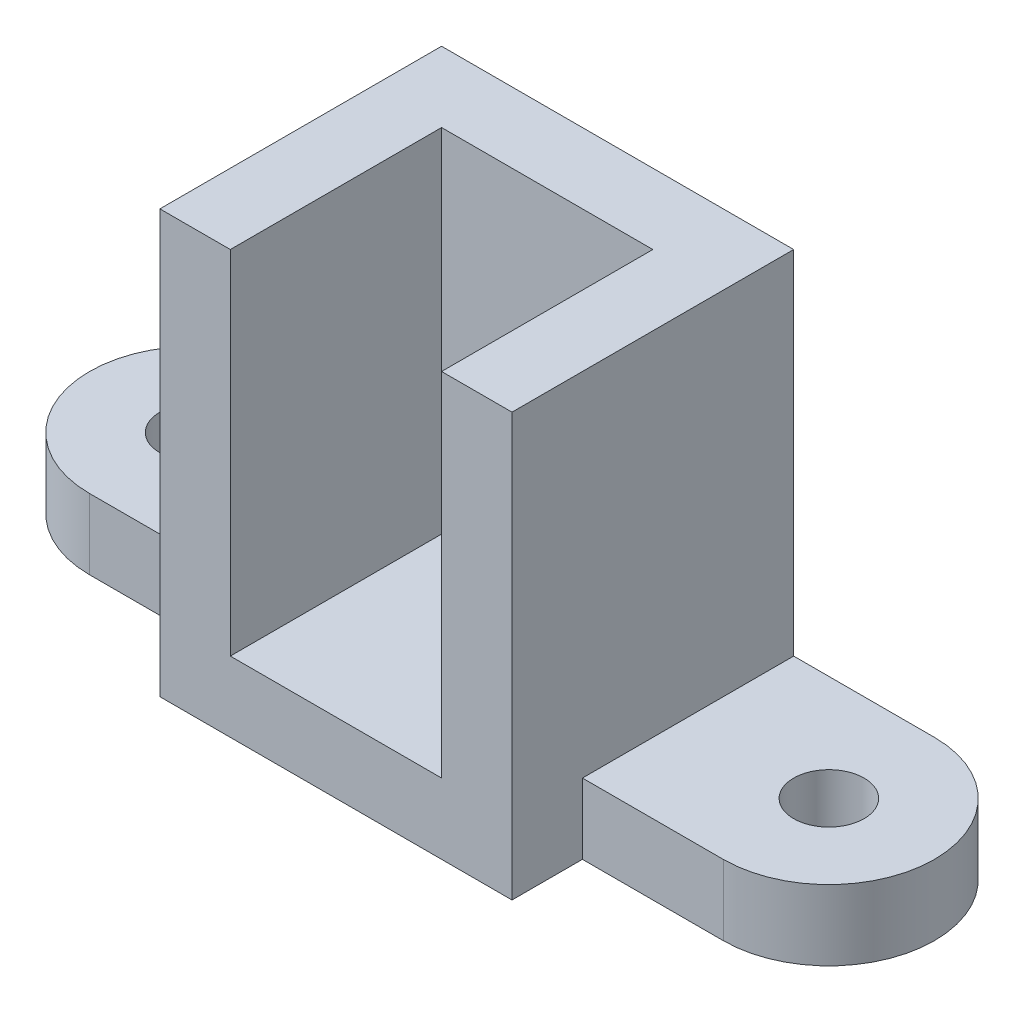
ISO-10303-21;
HEADER;
FILE_DESCRIPTION(('STEP AP214'),'2;1');
FILE_NAME('part.step','',(''),(''),'','','');
FILE_SCHEMA(('AUTOMOTIVE_DESIGN { 1 0 10303 214 1 1 1 1 }'));
ENDSEC;
DATA;
#1=APPLICATION_CONTEXT('core data for automotive mechanical design processes');
#2=APPLICATION_PROTOCOL_DEFINITION('international standard','automotive_design',2000,#1);
#3=PRODUCT_CONTEXT('',#1,'mechanical');
#4=PRODUCT('Part','Part','',(#3));
#5=PRODUCT_RELATED_PRODUCT_CATEGORY('part','',(#4));
#6=PRODUCT_DEFINITION_FORMATION('','',#4);
#7=PRODUCT_DEFINITION_CONTEXT('part definition',#1,'design');
#8=PRODUCT_DEFINITION('design','',#6,#7);
#9=PRODUCT_DEFINITION_SHAPE('','',#8);
#10=(LENGTH_UNIT() NAMED_UNIT(*) SI_UNIT(.MILLI.,.METRE.));
#11=(NAMED_UNIT(*) PLANE_ANGLE_UNIT() SI_UNIT($,.RADIAN.));
#12=(NAMED_UNIT(*) SI_UNIT($,.STERADIAN.) SOLID_ANGLE_UNIT());
#13=UNCERTAINTY_MEASURE_WITH_UNIT(LENGTH_MEASURE(1.E-05),#10,'distance_accuracy_value','');
#14=(GEOMETRIC_REPRESENTATION_CONTEXT(3) GLOBAL_UNCERTAINTY_ASSIGNED_CONTEXT((#13)) GLOBAL_UNIT_ASSIGNED_CONTEXT((#10,
#11,#12)) REPRESENTATION_CONTEXT('',''));
#15=CARTESIAN_POINT('',(0.,0.,0.));
#16=DIRECTION('',(0.,0.,1.));
#17=DIRECTION('',(1.,0.,0.));
#18=AXIS2_PLACEMENT_3D('',#15,#16,#17);
#19=CARTESIAN_POINT('',(0.,10.,-10.));
#20=DIRECTION('',(0.,0.,1.));
#21=DIRECTION('',(1.,0.,0.));
#22=AXIS2_PLACEMENT_3D('',#19,#20,#21);
#23=PLANE('',#22);
#24=DIRECTION('',(-1.,0.,0.));
#25=VECTOR('',#24,1.);
#26=CARTESIAN_POINT('',(0.,0.,-10.));
#27=LINE('',#26,#25);
#28=CARTESIAN_POINT('',(70.,0.,-10.));
#29=VERTEX_POINT('',#28);
#30=CARTESIAN_POINT('',(50.,0.,-10.));
#31=VERTEX_POINT('',#30);
#32=EDGE_CURVE('E217',#29,#31,#27,.T.);
#33=ORIENTED_EDGE('',*,*,#32,.F.);
#34=DIRECTION('',(0.,-1.,0.));
#35=VECTOR('',#34,1.);
#36=CARTESIAN_POINT('',(70.,10.,-10.));
#37=LINE('',#36,#35);
#38=CARTESIAN_POINT('',(70.,10.,-10.));
#39=VERTEX_POINT('',#38);
#40=EDGE_CURVE('E11',#39,#29,#37,.T.);
#41=ORIENTED_EDGE('',*,*,#40,.F.);
#42=DIRECTION('',(-1.,0.,0.));
#43=VECTOR('',#42,1.);
#44=CARTESIAN_POINT('',(0.,10.,-10.));
#45=LINE('',#44,#43);
#46=CARTESIAN_POINT('',(50.,10.,-10.));
#47=VERTEX_POINT('',#46);
#48=EDGE_CURVE('E204',#39,#47,#45,.T.);
#49=ORIENTED_EDGE('',*,*,#48,.T.);
#50=DIRECTION('',(0.,-1.,0.));
#51=VECTOR('',#50,1.);
#52=CARTESIAN_POINT('',(50.,10.,-10.));
#53=LINE('',#52,#51);
#54=EDGE_CURVE('E214',#47,#31,#53,.T.);
#55=ORIENTED_EDGE('',*,*,#54,.T.);
#56=EDGE_LOOP('',(#33,#41,#49,#55));
#57=FACE_BOUND('',#56,.T.);
#58=ADVANCED_FACE('F41',(#57),#23,.T.);
#59=CARTESIAN_POINT('',(70.,10.,-25.));
#60=DIRECTION('',(0.,-1.,0.));
#61=DIRECTION('',(0.,0.,-1.));
#62=AXIS2_PLACEMENT_3D('',#59,#60,#61);
#63=CYLINDRICAL_SURFACE('',#62,15.);
#64=CARTESIAN_POINT('',(70.,0.,-25.));
#65=DIRECTION('',(0.,1.,0.));
#66=DIRECTION('',(0.,0.,1.));
#67=AXIS2_PLACEMENT_3D('',#64,#65,#66);
#68=CIRCLE('',#67,15.);
#69=CARTESIAN_POINT('',(70.,0.,-40.));
#70=VERTEX_POINT('',#69);
#71=EDGE_CURVE('E222',#29,#70,#68,.T.);
#72=ORIENTED_EDGE('',*,*,#71,.T.);
#73=DIRECTION('',(0.,-1.,0.));
#74=VECTOR('',#73,1.);
#75=CARTESIAN_POINT('',(70.,10.,-40.));
#76=LINE('',#75,#74);
#77=CARTESIAN_POINT('',(70.,10.,-40.));
#78=VERTEX_POINT('',#77);
#79=EDGE_CURVE('E47',#78,#70,#76,.T.);
#80=ORIENTED_EDGE('',*,*,#79,.F.);
#81=CARTESIAN_POINT('',(70.,10.,-25.));
#82=DIRECTION('',(0.,1.,0.));
#83=DIRECTION('',(0.,0.,1.));
#84=AXIS2_PLACEMENT_3D('',#81,#82,#83);
#85=CIRCLE('',#84,15.);
#86=EDGE_CURVE('E210',#39,#78,#85,.T.);
#87=ORIENTED_EDGE('',*,*,#86,.F.);
#88=ORIENTED_EDGE('',*,*,#40,.T.);
#89=EDGE_LOOP('',(#72,#80,#87,#88));
#90=FACE_BOUND('',#89,.T.);
#91=ADVANCED_FACE('F232',(#90),#63,.T.);
#92=CARTESIAN_POINT('',(0.,10.,-40.));
#93=DIRECTION('',(0.,0.,-1.));
#94=DIRECTION('',(-1.,0.,0.));
#95=AXIS2_PLACEMENT_3D('',#92,#93,#94);
#96=PLANE('',#95);
#97=DIRECTION('',(1.,0.,0.));
#98=VECTOR('',#97,1.);
#99=CARTESIAN_POINT('',(0.,0.,-40.));
#100=LINE('',#99,#98);
#101=CARTESIAN_POINT('',(-20.,0.,-40.));
#102=VERTEX_POINT('',#101);
#103=EDGE_CURVE('E202',#102,#70,#100,.T.);
#104=ORIENTED_EDGE('',*,*,#103,.F.);
#105=DIRECTION('',(0.,-1.,0.));
#106=VECTOR('',#105,1.);
#107=CARTESIAN_POINT('',(-20.,10.,-40.));
#108=LINE('',#107,#106);
#109=CARTESIAN_POINT('',(-20.,10.,-40.));
#110=VERTEX_POINT('',#109);
#111=EDGE_CURVE('E260',#110,#102,#108,.T.);
#112=ORIENTED_EDGE('',*,*,#111,.F.);
#113=DIRECTION('',(-1.,0.,0.));
#114=VECTOR('',#113,1.);
#115=CARTESIAN_POINT('',(0.,10.,-40.));
#116=LINE('',#115,#114);
#117=CARTESIAN_POINT('',(0.,10.,-40.));
#118=VERTEX_POINT('',#117);
#119=EDGE_CURVE('E277',#118,#110,#116,.T.);
#120=ORIENTED_EDGE('',*,*,#119,.F.);
#121=DIRECTION('',(0.,-1.,0.));
#122=VECTOR('',#121,1.);
#123=CARTESIAN_POINT('',(0.,60.,-40.));
#124=LINE('',#123,#122);
#125=CARTESIAN_POINT('',(0.,60.,-40.));
#126=VERTEX_POINT('',#125);
#127=EDGE_CURVE('E191',#126,#118,#124,.T.);
#128=ORIENTED_EDGE('',*,*,#127,.F.);
#129=DIRECTION('',(1.,0.,0.));
#130=VECTOR('',#129,1.);
#131=CARTESIAN_POINT('',(0.,60.,-40.));
#132=LINE('',#131,#130);
#133=CARTESIAN_POINT('',(50.,60.,-40.));
#134=VERTEX_POINT('',#133);
#135=EDGE_CURVE('E172',#126,#134,#132,.T.);
#136=ORIENTED_EDGE('',*,*,#135,.T.);
#137=DIRECTION('',(0.,-1.,0.));
#138=VECTOR('',#137,1.);
#139=CARTESIAN_POINT('',(50.,60.,-40.));
#140=LINE('',#139,#138);
#141=CARTESIAN_POINT('',(50.,10.,-40.));
#142=VERTEX_POINT('',#141);
#143=EDGE_CURVE('E192',#134,#142,#140,.T.);
#144=ORIENTED_EDGE('',*,*,#143,.T.);
#145=DIRECTION('',(1.,0.,0.));
#146=VECTOR('',#145,1.);
#147=CARTESIAN_POINT('',(0.,10.,-40.));
#148=LINE('',#147,#146);
#149=EDGE_CURVE('E207',#142,#78,#148,.T.);
#150=ORIENTED_EDGE('',*,*,#149,.T.);
#151=ORIENTED_EDGE('',*,*,#79,.T.);
#152=EDGE_LOOP('',(#104,#112,#120,#128,#136,#144,#150,#151));
#153=FACE_BOUND('',#152,.T.);
#154=ADVANCED_FACE('F228',(#153),#96,.T.);
#155=CARTESIAN_POINT('',(70.,10.,-25.));
#156=DIRECTION('',(0.,-1.,0.));
#157=DIRECTION('',(0.,0.,-1.));
#158=AXIS2_PLACEMENT_3D('',#155,#156,#157);
#159=CYLINDRICAL_SURFACE('',#158,5.);
#160=CARTESIAN_POINT('',(70.,10.,-25.));
#161=DIRECTION('',(0.,1.,0.));
#162=DIRECTION('',(0.,0.,1.));
#163=AXIS2_PLACEMENT_3D('',#160,#161,#162);
#164=CIRCLE('',#163,5.);
#165=CARTESIAN_POINT('',(70.,10.,-20.));
#166=VERTEX_POINT('',#165);
#167=EDGE_CURVE('E203',#166,#166,#164,.T.);
#168=ORIENTED_EDGE('',*,*,#167,.T.);
#169=EDGE_LOOP('',(#168));
#170=FACE_BOUND('',#169,.T.);
#171=CARTESIAN_POINT('',(70.,0.,-25.));
#172=DIRECTION('',(0.,1.,0.));
#173=DIRECTION('',(0.,0.,1.));
#174=AXIS2_PLACEMENT_3D('',#171,#172,#173);
#175=CIRCLE('',#174,5.);
#176=CARTESIAN_POINT('',(70.,0.,-20.));
#177=VERTEX_POINT('',#176);
#178=EDGE_CURVE('E199',#177,#177,#175,.T.);
#179=ORIENTED_EDGE('',*,*,#178,.F.);
#180=EDGE_LOOP('',(#179));
#181=FACE_BOUND('',#180,.T.);
#182=ADVANCED_FACE('F43',(#170,#181),#159,.F.);
#183=CARTESIAN_POINT('',(0.,10.,0.));
#184=DIRECTION('',(0.,1.,0.));
#185=DIRECTION('',(0.,0.,1.));
#186=AXIS2_PLACEMENT_3D('',#183,#184,#185);
#187=PLANE('',#186);
#188=ORIENTED_EDGE('',*,*,#167,.F.);
#189=EDGE_LOOP('',(#188));
#190=FACE_BOUND('',#189,.T.);
#191=ORIENTED_EDGE('',*,*,#48,.F.);
#192=ORIENTED_EDGE('',*,*,#86,.T.);
#193=ORIENTED_EDGE('',*,*,#149,.F.);
#194=DIRECTION('',(0.,0.,-1.));
#195=VECTOR('',#194,1.);
#196=CARTESIAN_POINT('',(50.,10.,0.));
#197=LINE('',#196,#195);
#198=EDGE_CURVE('E215',#47,#142,#197,.T.);
#199=ORIENTED_EDGE('',*,*,#198,.F.);
#200=EDGE_LOOP('',(#191,#192,#193,#199));
#201=FACE_BOUND('',#200,.T.);
#202=ADVANCED_FACE('F287',(#190,#201),#187,.T.);
#203=CARTESIAN_POINT('',(0.,0.,0.));
#204=DIRECTION('',(0.,1.,0.));
#205=DIRECTION('',(0.,0.,1.));
#206=AXIS2_PLACEMENT_3D('',#203,#204,#205);
#207=PLANE('',#206);
#208=ORIENTED_EDGE('',*,*,#178,.T.);
#209=EDGE_LOOP('',(#208));
#210=FACE_BOUND('',#209,.T.);
#211=ORIENTED_EDGE('',*,*,#32,.T.);
#212=DIRECTION('',(0.,0.,-1.));
#213=VECTOR('',#212,1.);
#214=CARTESIAN_POINT('',(50.,0.,0.));
#215=LINE('',#214,#213);
#216=CARTESIAN_POINT('',(50.,0.,0.));
#217=VERTEX_POINT('',#216);
#218=EDGE_CURVE('E183',#217,#31,#215,.T.);
#219=ORIENTED_EDGE('',*,*,#218,.F.);
#220=DIRECTION('',(1.,0.,0.));
#221=VECTOR('',#220,1.);
#222=CARTESIAN_POINT('',(0.,0.,0.));
#223=LINE('',#222,#221);
#224=CARTESIAN_POINT('',(0.,0.,0.));
#225=VERTEX_POINT('',#224);
#226=EDGE_CURVE('E185',#225,#217,#223,.T.);
#227=ORIENTED_EDGE('',*,*,#226,.F.);
#228=DIRECTION('',(0.,0.,-1.));
#229=VECTOR('',#228,1.);
#230=CARTESIAN_POINT('',(0.,0.,0.));
#231=LINE('',#230,#229);
#232=CARTESIAN_POINT('',(0.,0.,-10.));
#233=VERTEX_POINT('',#232);
#234=EDGE_CURVE('E173',#225,#233,#231,.T.);
#235=ORIENTED_EDGE('',*,*,#234,.T.);
#236=DIRECTION('',(1.,0.,0.));
#237=VECTOR('',#236,1.);
#238=CARTESIAN_POINT('',(0.,0.,-10.));
#239=LINE('',#238,#237);
#240=CARTESIAN_POINT('',(-20.,0.,-10.));
#241=VERTEX_POINT('',#240);
#242=EDGE_CURVE('E64',#241,#233,#239,.T.);
#243=ORIENTED_EDGE('',*,*,#242,.F.);
#244=CARTESIAN_POINT('',(-20.,0.,-25.));
#245=DIRECTION('',(0.,1.,0.));
#246=DIRECTION('',(0.,0.,1.));
#247=AXIS2_PLACEMENT_3D('',#244,#245,#246);
#248=CIRCLE('',#247,15.);
#249=EDGE_CURVE('E242',#241,#102,#248,.F.);
#250=ORIENTED_EDGE('',*,*,#249,.T.);
#251=ORIENTED_EDGE('',*,*,#103,.T.);
#252=ORIENTED_EDGE('',*,*,#71,.F.);
#253=EDGE_LOOP('',(#211,#219,#227,#235,#243,#250,#251,#252));
#254=FACE_BOUND('',#253,.T.);
#255=CARTESIAN_POINT('',(-20.,0.,-25.));
#256=DIRECTION('',(0.,1.,0.));
#257=DIRECTION('',(0.,0.,1.));
#258=AXIS2_PLACEMENT_3D('',#255,#256,#257);
#259=CIRCLE('',#258,5.);
#260=CARTESIAN_POINT('',(-20.,0.,-20.));
#261=VERTEX_POINT('',#260);
#262=EDGE_CURVE('E241',#261,#261,#259,.F.);
#263=ORIENTED_EDGE('',*,*,#262,.F.);
#264=EDGE_LOOP('',(#263));
#265=FACE_BOUND('',#264,.T.);
#266=ADVANCED_FACE('F236',(#210,#254,#265),#207,.F.);
#267=CARTESIAN_POINT('',(0.,60.,0.));
#268=DIRECTION('',(0.,0.,-1.));
#269=DIRECTION('',(-1.,0.,0.));
#270=AXIS2_PLACEMENT_3D('',#267,#268,#269);
#271=PLANE('',#270);
#272=DIRECTION('',(1.,0.,0.));
#273=VECTOR('',#272,1.);
#274=CARTESIAN_POINT('',(0.,60.,0.));
#275=LINE('',#274,#273);
#276=CARTESIAN_POINT('',(40.,60.,0.));
#277=VERTEX_POINT('',#276);
#278=CARTESIAN_POINT('',(50.,60.,0.));
#279=VERTEX_POINT('',#278);
#280=EDGE_CURVE('E166',#277,#279,#275,.T.);
#281=ORIENTED_EDGE('',*,*,#280,.F.);
#282=DIRECTION('',(0.,-1.,0.));
#283=VECTOR('',#282,1.);
#284=CARTESIAN_POINT('',(40.,60.,0.));
#285=LINE('',#284,#283);
#286=CARTESIAN_POINT('',(40.,10.,0.));
#287=VERTEX_POINT('',#286);
#288=EDGE_CURVE('E248',#277,#287,#285,.T.);
#289=ORIENTED_EDGE('',*,*,#288,.T.);
#290=DIRECTION('',(1.,0.,0.));
#291=VECTOR('',#290,1.);
#292=CARTESIAN_POINT('',(0.,10.,0.));
#293=LINE('',#292,#291);
#294=CARTESIAN_POINT('',(10.,10.,0.));
#295=VERTEX_POINT('',#294);
#296=EDGE_CURVE('E161',#295,#287,#293,.T.);
#297=ORIENTED_EDGE('',*,*,#296,.F.);
#298=DIRECTION('',(0.,-1.,0.));
#299=VECTOR('',#298,1.);
#300=CARTESIAN_POINT('',(10.,60.,0.));
#301=LINE('',#300,#299);
#302=CARTESIAN_POINT('',(10.,60.,0.));
#303=VERTEX_POINT('',#302);
#304=EDGE_CURVE('E148',#303,#295,#301,.T.);
#305=ORIENTED_EDGE('',*,*,#304,.F.);
#306=CARTESIAN_POINT('',(0.,60.,0.));
#307=VERTEX_POINT('',#306);
#308=EDGE_CURVE('E160',#307,#303,#275,.T.);
#309=ORIENTED_EDGE('',*,*,#308,.F.);
#310=DIRECTION('',(0.,-1.,0.));
#311=VECTOR('',#310,1.);
#312=CARTESIAN_POINT('',(0.,60.,0.));
#313=LINE('',#312,#311);
#314=EDGE_CURVE('E182',#307,#225,#313,.T.);
#315=ORIENTED_EDGE('',*,*,#314,.T.);
#316=ORIENTED_EDGE('',*,*,#226,.T.);
#317=DIRECTION('',(0.,-1.,0.));
#318=VECTOR('',#317,1.);
#319=CARTESIAN_POINT('',(50.,60.,0.));
#320=LINE('',#319,#318);
#321=EDGE_CURVE('E197',#279,#217,#320,.T.);
#322=ORIENTED_EDGE('',*,*,#321,.F.);
#323=EDGE_LOOP('',(#281,#289,#297,#305,#309,#315,#316,#322));
#324=FACE_BOUND('',#323,.T.);
#325=ADVANCED_FACE('F156',(#324),#271,.F.);
#326=CARTESIAN_POINT('',(50.,60.,0.));
#327=DIRECTION('',(-1.,0.,0.));
#328=DIRECTION('',(0.,0.,1.));
#329=AXIS2_PLACEMENT_3D('',#326,#327,#328);
#330=PLANE('',#329);
#331=ORIENTED_EDGE('',*,*,#54,.F.);
#332=ORIENTED_EDGE('',*,*,#198,.T.);
#333=ORIENTED_EDGE('',*,*,#143,.F.);
#334=DIRECTION('',(0.,0.,-1.));
#335=VECTOR('',#334,1.);
#336=CARTESIAN_POINT('',(50.,60.,0.));
#337=LINE('',#336,#335);
#338=EDGE_CURVE('E169',#279,#134,#337,.T.);
#339=ORIENTED_EDGE('',*,*,#338,.F.);
#340=ORIENTED_EDGE('',*,*,#321,.T.);
#341=ORIENTED_EDGE('',*,*,#218,.T.);
#342=EDGE_LOOP('',(#331,#332,#333,#339,#340,#341));
#343=FACE_BOUND('',#342,.T.);
#344=ADVANCED_FACE('F300',(#343),#330,.F.);
#345=CARTESIAN_POINT('',(0.,60.,0.));
#346=DIRECTION('',(-1.,0.,0.));
#347=DIRECTION('',(0.,0.,1.));
#348=AXIS2_PLACEMENT_3D('',#345,#346,#347);
#349=PLANE('',#348);
#350=DIRECTION('',(0.,0.,-1.));
#351=VECTOR('',#350,1.);
#352=CARTESIAN_POINT('',(0.,10.,0.));
#353=LINE('',#352,#351);
#354=CARTESIAN_POINT('',(0.,10.,-10.));
#355=VERTEX_POINT('',#354);
#356=EDGE_CURVE('E269',#355,#118,#353,.T.);
#357=ORIENTED_EDGE('',*,*,#356,.F.);
#358=DIRECTION('',(0.,-1.,0.));
#359=VECTOR('',#358,1.);
#360=CARTESIAN_POINT('',(0.,10.,-10.));
#361=LINE('',#360,#359);
#362=EDGE_CURVE('E256',#355,#233,#361,.T.);
#363=ORIENTED_EDGE('',*,*,#362,.T.);
#364=ORIENTED_EDGE('',*,*,#234,.F.);
#365=ORIENTED_EDGE('',*,*,#314,.F.);
#366=DIRECTION('',(0.,0.,-1.));
#367=VECTOR('',#366,1.);
#368=CARTESIAN_POINT('',(0.,60.,0.));
#369=LINE('',#368,#367);
#370=EDGE_CURVE('E170',#307,#126,#369,.T.);
#371=ORIENTED_EDGE('',*,*,#370,.T.);
#372=ORIENTED_EDGE('',*,*,#127,.T.);
#373=EDGE_LOOP('',(#357,#363,#364,#365,#371,#372));
#374=FACE_BOUND('',#373,.T.);
#375=ADVANCED_FACE('F330',(#374),#349,.T.);
#376=CARTESIAN_POINT('',(0.,60.,0.));
#377=DIRECTION('',(0.,1.,0.));
#378=DIRECTION('',(0.,0.,1.));
#379=AXIS2_PLACEMENT_3D('',#376,#377,#378);
#380=PLANE('',#379);
#381=DIRECTION('',(0.,0.,-1.));
#382=VECTOR('',#381,1.);
#383=CARTESIAN_POINT('',(40.,60.,0.));
#384=LINE('',#383,#382);
#385=CARTESIAN_POINT('',(40.,60.,-30.));
#386=VERTEX_POINT('',#385);
#387=EDGE_CURVE('E272',#277,#386,#384,.T.);
#388=ORIENTED_EDGE('',*,*,#387,.F.);
#389=ORIENTED_EDGE('',*,*,#280,.T.);
#390=ORIENTED_EDGE('',*,*,#338,.T.);
#391=ORIENTED_EDGE('',*,*,#135,.F.);
#392=ORIENTED_EDGE('',*,*,#370,.F.);
#393=ORIENTED_EDGE('',*,*,#308,.T.);
#394=DIRECTION('',(0.,0.,-1.));
#395=VECTOR('',#394,1.);
#396=CARTESIAN_POINT('',(10.,60.,0.));
#397=LINE('',#396,#395);
#398=CARTESIAN_POINT('',(10.,60.,-30.));
#399=VERTEX_POINT('',#398);
#400=EDGE_CURVE('E141',#303,#399,#397,.T.);
#401=ORIENTED_EDGE('',*,*,#400,.T.);
#402=DIRECTION('',(1.,0.,0.));
#403=VECTOR('',#402,1.);
#404=CARTESIAN_POINT('',(0.,60.,-30.));
#405=LINE('',#404,#403);
#406=EDGE_CURVE('E57',#399,#386,#405,.T.);
#407=ORIENTED_EDGE('',*,*,#406,.T.);
#408=EDGE_LOOP('',(#388,#389,#390,#391,#392,#393,#401,#407));
#409=FACE_BOUND('',#408,.T.);
#410=ADVANCED_FACE('F163',(#409),#380,.T.);
#411=CARTESIAN_POINT('',(-20.,10.,-25.));
#412=DIRECTION('',(0.,-1.,0.));
#413=DIRECTION('',(0.,0.,-1.));
#414=AXIS2_PLACEMENT_3D('',#411,#412,#413);
#415=CYLINDRICAL_SURFACE('',#414,15.);
#416=ORIENTED_EDGE('',*,*,#249,.F.);
#417=DIRECTION('',(0.,-1.,0.));
#418=VECTOR('',#417,1.);
#419=CARTESIAN_POINT('',(-20.,10.,-10.));
#420=LINE('',#419,#418);
#421=CARTESIAN_POINT('',(-20.,10.,-10.));
#422=VERTEX_POINT('',#421);
#423=EDGE_CURVE('E171',#422,#241,#420,.T.);
#424=ORIENTED_EDGE('',*,*,#423,.F.);
#425=CARTESIAN_POINT('',(-20.,10.,-25.));
#426=DIRECTION('',(0.,1.,0.));
#427=DIRECTION('',(0.,0.,1.));
#428=AXIS2_PLACEMENT_3D('',#425,#426,#427);
#429=CIRCLE('',#428,15.);
#430=EDGE_CURVE('E258',#422,#110,#429,.F.);
#431=ORIENTED_EDGE('',*,*,#430,.T.);
#432=ORIENTED_EDGE('',*,*,#111,.T.);
#433=EDGE_LOOP('',(#416,#424,#431,#432));
#434=FACE_BOUND('',#433,.T.);
#435=ADVANCED_FACE('F270',(#434),#415,.T.);
#436=CARTESIAN_POINT('',(0.,10.,-10.));
#437=DIRECTION('',(0.,0.,-1.));
#438=DIRECTION('',(-1.,0.,0.));
#439=AXIS2_PLACEMENT_3D('',#436,#437,#438);
#440=PLANE('',#439);
#441=ORIENTED_EDGE('',*,*,#242,.T.);
#442=ORIENTED_EDGE('',*,*,#362,.F.);
#443=DIRECTION('',(1.,0.,0.));
#444=VECTOR('',#443,1.);
#445=CARTESIAN_POINT('',(0.,10.,-10.));
#446=LINE('',#445,#444);
#447=EDGE_CURVE('E262',#422,#355,#446,.T.);
#448=ORIENTED_EDGE('',*,*,#447,.F.);
#449=ORIENTED_EDGE('',*,*,#423,.T.);
#450=EDGE_LOOP('',(#441,#442,#448,#449));
#451=FACE_BOUND('',#450,.T.);
#452=ADVANCED_FACE('F263',(#451),#440,.F.);
#453=CARTESIAN_POINT('',(-20.,10.,-25.));
#454=DIRECTION('',(0.,-1.,0.));
#455=DIRECTION('',(0.,0.,-1.));
#456=AXIS2_PLACEMENT_3D('',#453,#454,#455);
#457=CYLINDRICAL_SURFACE('',#456,5.);
#458=CARTESIAN_POINT('',(-20.,10.,-25.));
#459=DIRECTION('',(0.,1.,0.));
#460=DIRECTION('',(0.,0.,1.));
#461=AXIS2_PLACEMENT_3D('',#458,#459,#460);
#462=CIRCLE('',#461,5.);
#463=CARTESIAN_POINT('',(-20.,10.,-20.));
#464=VERTEX_POINT('',#463);
#465=EDGE_CURVE('E253',#464,#464,#462,.F.);
#466=ORIENTED_EDGE('',*,*,#465,.F.);
#467=EDGE_LOOP('',(#466));
#468=FACE_BOUND('',#467,.T.);
#469=ORIENTED_EDGE('',*,*,#262,.T.);
#470=EDGE_LOOP('',(#469));
#471=FACE_BOUND('',#470,.T.);
#472=ADVANCED_FACE('F283',(#468,#471),#457,.F.);
#473=CARTESIAN_POINT('',(0.,10.,0.));
#474=DIRECTION('',(0.,1.,0.));
#475=DIRECTION('',(0.,0.,1.));
#476=AXIS2_PLACEMENT_3D('',#473,#474,#475);
#477=PLANE('',#476);
#478=ORIENTED_EDGE('',*,*,#430,.F.);
#479=ORIENTED_EDGE('',*,*,#447,.T.);
#480=ORIENTED_EDGE('',*,*,#356,.T.);
#481=ORIENTED_EDGE('',*,*,#119,.T.);
#482=EDGE_LOOP('',(#478,#479,#480,#481));
#483=FACE_BOUND('',#482,.T.);
#484=ORIENTED_EDGE('',*,*,#465,.T.);
#485=EDGE_LOOP('',(#484));
#486=FACE_BOUND('',#485,.T.);
#487=ADVANCED_FACE('F282',(#483,#486),#477,.T.);
#488=CARTESIAN_POINT('',(0.,10.,-30.));
#489=DIRECTION('',(0.,0.,-1.));
#490=DIRECTION('',(-1.,0.,0.));
#491=AXIS2_PLACEMENT_3D('',#488,#489,#490);
#492=PLANE('',#491);
#493=DIRECTION('',(0.,-1.,0.));
#494=VECTOR('',#493,1.);
#495=CARTESIAN_POINT('',(40.,60.,-30.));
#496=LINE('',#495,#494);
#497=CARTESIAN_POINT('',(40.,10.,-30.));
#498=VERTEX_POINT('',#497);
#499=EDGE_CURVE('E328',#386,#498,#496,.T.);
#500=ORIENTED_EDGE('',*,*,#499,.F.);
#501=ORIENTED_EDGE('',*,*,#406,.F.);
#502=DIRECTION('',(0.,-1.,0.));
#503=VECTOR('',#502,1.);
#504=CARTESIAN_POINT('',(10.,60.,-30.));
#505=LINE('',#504,#503);
#506=CARTESIAN_POINT('',(10.,10.,-30.));
#507=VERTEX_POINT('',#506);
#508=EDGE_CURVE('E146',#399,#507,#505,.T.);
#509=ORIENTED_EDGE('',*,*,#508,.T.);
#510=DIRECTION('',(1.,0.,0.));
#511=VECTOR('',#510,1.);
#512=CARTESIAN_POINT('',(0.,10.,-30.));
#513=LINE('',#512,#511);
#514=EDGE_CURVE('E243',#507,#498,#513,.T.);
#515=ORIENTED_EDGE('',*,*,#514,.T.);
#516=EDGE_LOOP('',(#500,#501,#509,#515));
#517=FACE_BOUND('',#516,.T.);
#518=ADVANCED_FACE('F336',(#517),#492,.F.);
#519=CARTESIAN_POINT('',(0.,10.,0.));
#520=DIRECTION('',(0.,1.,0.));
#521=DIRECTION('',(0.,0.,1.));
#522=AXIS2_PLACEMENT_3D('',#519,#520,#521);
#523=PLANE('',#522);
#524=ORIENTED_EDGE('',*,*,#514,.F.);
#525=DIRECTION('',(0.,0.,-1.));
#526=VECTOR('',#525,1.);
#527=CARTESIAN_POINT('',(10.,10.,0.));
#528=LINE('',#527,#526);
#529=EDGE_CURVE('E337',#295,#507,#528,.T.);
#530=ORIENTED_EDGE('',*,*,#529,.F.);
#531=ORIENTED_EDGE('',*,*,#296,.T.);
#532=DIRECTION('',(0.,0.,-1.));
#533=VECTOR('',#532,1.);
#534=CARTESIAN_POINT('',(40.,10.,0.));
#535=LINE('',#534,#533);
#536=EDGE_CURVE('E334',#287,#498,#535,.T.);
#537=ORIENTED_EDGE('',*,*,#536,.T.);
#538=EDGE_LOOP('',(#524,#530,#531,#537));
#539=FACE_BOUND('',#538,.T.);
#540=ADVANCED_FACE('F345',(#539),#523,.T.);
#541=CARTESIAN_POINT('',(40.,60.,0.));
#542=DIRECTION('',(-1.,0.,0.));
#543=DIRECTION('',(0.,0.,1.));
#544=AXIS2_PLACEMENT_3D('',#541,#542,#543);
#545=PLANE('',#544);
#546=ORIENTED_EDGE('',*,*,#536,.F.);
#547=ORIENTED_EDGE('',*,*,#288,.F.);
#548=ORIENTED_EDGE('',*,*,#387,.T.);
#549=ORIENTED_EDGE('',*,*,#499,.T.);
#550=EDGE_LOOP('',(#546,#547,#548,#549));
#551=FACE_BOUND('',#550,.T.);
#552=ADVANCED_FACE('F343',(#551),#545,.T.);
#553=CARTESIAN_POINT('',(10.,60.,0.));
#554=DIRECTION('',(-1.,0.,0.));
#555=DIRECTION('',(0.,0.,1.));
#556=AXIS2_PLACEMENT_3D('',#553,#554,#555);
#557=PLANE('',#556);
#558=ORIENTED_EDGE('',*,*,#508,.F.);
#559=ORIENTED_EDGE('',*,*,#400,.F.);
#560=ORIENTED_EDGE('',*,*,#304,.T.);
#561=ORIENTED_EDGE('',*,*,#529,.T.);
#562=EDGE_LOOP('',(#558,#559,#560,#561));
#563=FACE_BOUND('',#562,.T.);
#564=ADVANCED_FACE('F144',(#563),#557,.F.);
#565=CLOSED_SHELL('',(#58,#91,#154,#182,#202,#266,#325,#344,#375,#410,#435,#452,#472,#487,#518,
#540,#552,#564));
#566=MANIFOLD_SOLID_BREP('B2',#565);
#567=ADVANCED_BREP_SHAPE_REPRESENTATION('',(#18,#566),#14);
#568=SHAPE_DEFINITION_REPRESENTATION(#9,#567);
ENDSEC;
END-ISO-10303-21;
